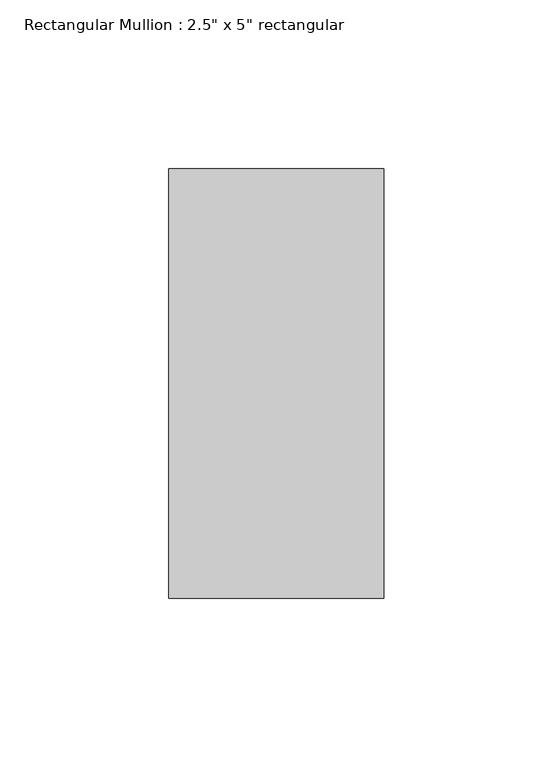
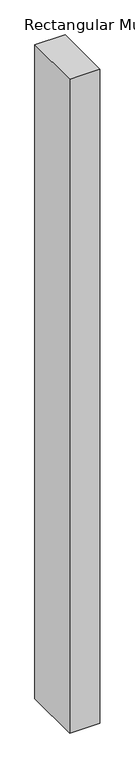
"""IFC4 building model written with IfcOpenShell, lengths in millimetres: member geometry."""

from ifc_helpers import new_model, si_unit, frame, origin, place, context, project, spatial, polyline, outline, extrude, source, transform, mapped, element, save


def member_f11946c0(model_context):
    return source(origin(), model_context, "Body", "SweptSolid", [
        extrude(outline(polyline([(0.0, 63.5), (0.0, -63.5), (-63.5, -63.5), (-63.5, 63.5), (0.0, 63.5)])), frame((0.0, 0.0, -1458.2177433), z_axis=(0.0, 0.0, 1.0), x_axis=(1.0, 0.0, 0.0)), (0.0, 0.0, 1.0), 1458.2177433),
    ])


if __name__ == "__main__":
    model = new_model("IFC4")
    model_context = context("Model", 3, world=origin())
    ifc_project = project(units=[si_unit("LENGTHUNIT", "METRE", prefix="MILLI")], contexts=[model_context])
    site = spatial("IfcSite", under=ifc_project)
    building = spatial("IfcBuilding", under=site)
    placement = place(None, origin())
    member_shape = member_f11946c0(model_context)
    element("IfcMember", 1, ObjectType="Rectangular Mullion : 2.5\" x 5\" rectangular", at=placement, inside=building, context=model_context, shape_type="MappedRepresentation", body=[
        mapped(member_shape, transform((0.0, 0.0, 0.0), x_axis=(1.0, 0.0, 0.0), y_axis=(0.0, 1.0, 0.0), z_axis=(0.0, 0.0, 1.0))),
    ])
    save(model, "model.ifc")

# Revit data of these elements
# Type "Rectangular Mullion : 2.5\" x 5\" rectangular"
#   built-in parameter 1007304 = 0.416667 (stored number, unit not read)
#   built-in parameter 1007301 = 0.104167 (stored number, unit not read)
#   built-in parameter 1007300 = 0.104167 (stored number, unit not read)
# Element 1 (IfcMember, "Rectangular Mullion : 2.5\" x 5\" rectangular")
#   Materials on its faces: "Iron, Ductile"
# Materials
#   "Iron, Ductile": class "Metal", colour RGB 0 0 0, transparency 0, Description = "Ductile cast iron", Cost = 0
